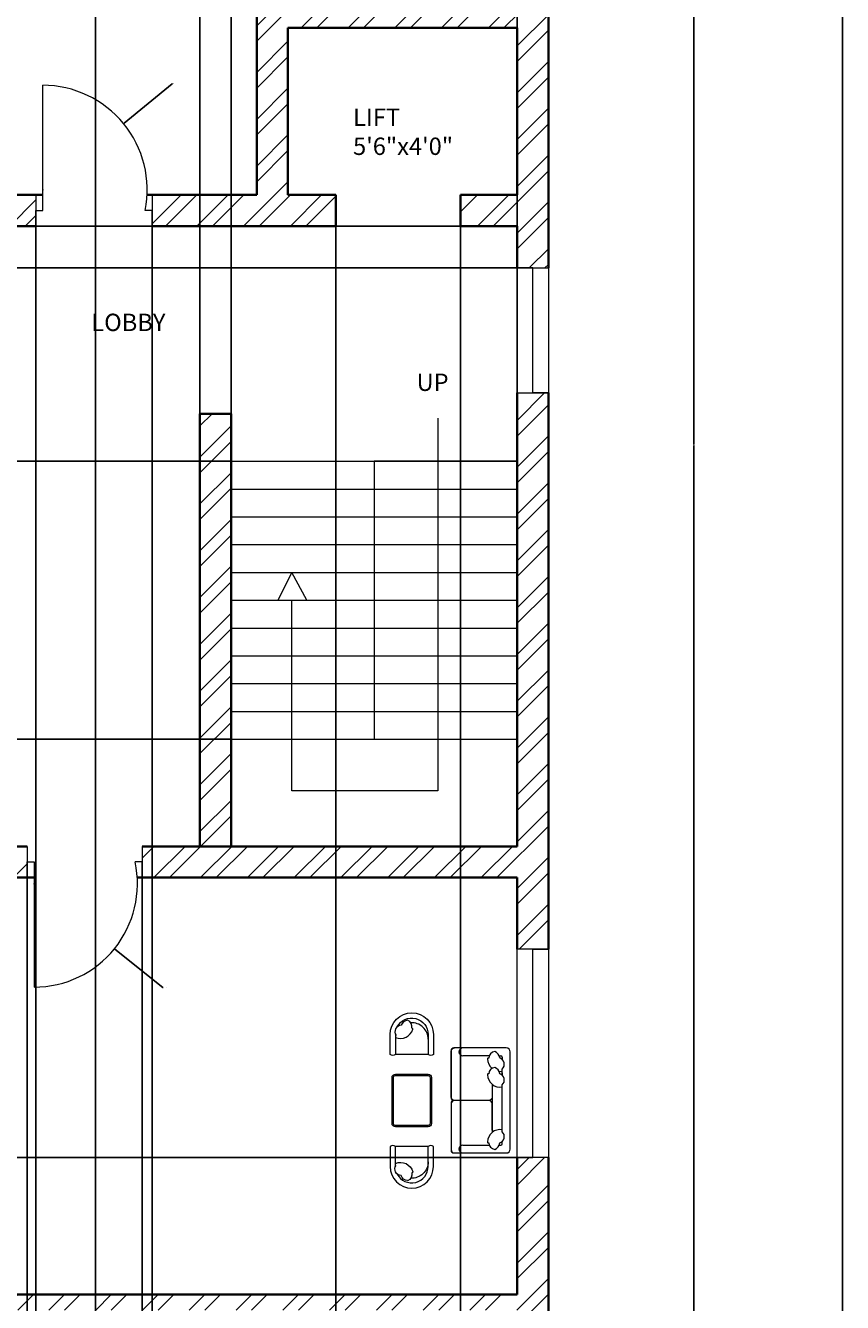
# Model space of a CAD drawing. Units: inches. Extents: x 1748 to 2382, y 1346 to 2284.
# Tile 16 of 26: x 2147 to 2382, y 1604 to 1971. Entities that reach past the tile are written whole.
import ezdxf

# ---------------------------------------------------------------- set-up
doc = ezdxf.new("R2010")
doc.units = ezdxf.units.IN
for name, color, linetype, lineweight in [('A-ANNO-DIMS', 2, 'Continuous', 18), ('A-ANNO-SYMB', 60, 'Continuous', 18), ('A-ANNO-TTLB', 7, 'Continuous', 25), ('A-AREA-IDEN', 7, 'Continuous', 18), ('A-DOOR', 21, 'Continuous', 18), ('A-FLOR-STRS', 60, 'Continuous', 18), ('A-FURN', 8, 'Continuous', 13), ('A-GLAZ', 191, 'Continuous', 18), ('A-WALL', 7, 'Continuous', 35), ('A-WALL-PATT', 9, 'Continuous', 13)]:
    doc.layers.add(name, color=color, linetype=linetype, lineweight=lineweight)
doc.styles.get("Standard").update_dxf_attribs({"font": 'arial.ttf'})
doc.dimstyles.get("Standard").update_dxf_attribs({"dimtxt": 0.18, "dimasz": 0.18, "dimexe": 0.18, "dimexo": 0.0625, "dimgap": 0.09, "dimtad": 0, "dimtih": 1, "dimtoh": 1, "dimdec": 4, "dimzin": 0, "dimdsep": 46, "dimtxsty": 'Standard', "dimcen": 0.09, "dimadec": 0, "dimazin": 0, "dimtfac": 1, "dimtdec": 4, "dimtofl": 0, "dimtmove": 0, "dimatfit": 3, "dimfxl": 1, "dimtolj": 1, "dimtzin": 0, "dimarcsym": 0})

# ---------------------------------------------------------------- blocks, each defined once
blk = doc.blocks.new('A$C1352')
at = {"color": 0}
for points in [[(0.003, 0.053), (0.003, 0.553, -0.414214), (0.053, 0.603), (0.753, 0.603, -0.414214), (0.803, 0.553), (0.803, 0.053, -0.414214), (0.753, 0.003), (0.053, 0.003, -0.414214)], [(0.023, 0.053), (0.023, 0.553, -0.414214), (0.053, 0.583), (0.753, 0.583, -0.414214), (0.783, 0.553), (0.783, 0.053, -0.414214), (0.753, 0.023), (0.053, 0.023, -0.414214)]]:
    blk.add_lwpolyline(points, format="xyb", close=True, dxfattribs=at)
blk = doc.blocks.new('WIN-60-DEEP')
for p, q in [((0, 9), (0, 0)), ((60, 9), (0, 9)), ((60, 4.5), (60, 9)), ((60, 9), (60, 0)), ((0, 0), (0, 4.5)), ((0, 4.5), (60, 4.5)), ((0, 0), (60, 0))]:
    blk.add_line(p, q)
blk = doc.blocks.new('WIN-36-DEEP')
for p, q in [((0, 9), (0, 0)), ((0, 9), (36, 9)), ((36, 4.5), (36, 9)), ((36, 9), (36, 0)), ((0, 0), (0, 4.5)), ((0, 4.5), (36, 4.5)), ((36, 0), (0, 0))]:
    blk.add_line(p, q)
blk = doc.blocks.new('CHAIR-LOUNGE')
blk.add_line((1.52, 6.05), (1.51, 0.29))
at = {"ltscale": 0.03}
blk.add_lwpolyline([(1.51, 0.29, -0.369229), (0, 0.29), (0.01, 6.05, -1), (12.48, 6.04), (12.47, 0.28, -0.369229), (10.96, 0.28)], format="xyb", close=True, dxfattribs=at)
blk.add_lwpolyline([(2.05, 8.23, -0.785087), (10.96, 6.04), (10.96, 0.28)], format="xyb")
for centre, radius, start, end in [((3.29, 6.8), 1.89, 92.9922, 214.1401), ((3, 8.54), 3.66, 247.0143, 344.2857), ((5.21, 8.01), 2.13, 94.9999, 161.3534), ((4.35, 8.32), 1.94, 346.6403, 69.4695), ((6.24, 4.71), 4.72, 359.9461, 93.658), ((6.33, 7.66), 0.226, 330.6238, 113.7423), ((6.24, 6.05), 4.72, 178.8536, 179.9461)]:
    blk.add_arc(centre, radius, start, end)
blk = doc.blocks.new('*D35')
at = {"layer": 'A-ANNO-DIMS', "color": 0, "lineweight": -2, "transparency": 16777216}
for p, q in [((2297.52, 2232.85), (2339.54, 2232.85)), ((2339.36, 2232.67), (2339.36, 1850.53)), ((2339.36, 1468.03), (2339.36, 1850.17)), ((2297.52, 1467.85), (2339.54, 1467.85))]:
    blk.add_line(p, q, dxfattribs=at)
at = {"layer": 'A-ANNO-DIMS', "color": 0, "transparency": 16777216}
for points in [[(2339.33, 2232.67), (2339.39, 2232.67), (2339.36, 2232.85)], [(2339.33, 1468.03), (2339.39, 1468.03), (2339.36, 1467.85)]]:
    blk.add_solid(points, dxfattribs=at)
at = {"layer": 'Defpoints', "color": 0, "transparency": 16777216}
for p in [(2297.46, 2232.85), (2339.36, 2232.85), (2297.46, 1467.85)]:
    blk.add_point(p, dxfattribs=at)
at = {"layer": 'A-ANNO-DIMS', "color": 0, "transparency": 16777216, "insert": (2339.36, 1850.35), "char_height": 0.18, "attachment_point": 5}
blk.add_mtext('\\A1;765', dxfattribs=at)
blk = doc.blocks.new('*D39')
at = {"layer": 'A-ANNO-DIMS', "color": 0, "lineweight": -2, "transparency": 16777216}
for p, q in [((2139.96, 1734.91), (2139.96, 2274.93)), ((2140.14, 2274.75), (2168.14, 2274.75)), ((2196.89, 2274.75), (2168.89, 2274.75)), ((2197.07, 1734.91), (2197.07, 2274.93))]:
    blk.add_line(p, q, dxfattribs=at)
at = {"layer": 'A-ANNO-DIMS', "color": 0, "transparency": 16777216}
for points in [[(2140.14, 2274.78), (2140.14, 2274.72), (2139.96, 2274.75)], [(2196.89, 2274.78), (2196.89, 2274.72), (2197.07, 2274.75)]]:
    blk.add_solid(points, dxfattribs=at)
at = {"layer": 'Defpoints', "color": 0, "transparency": 16777216}
for p in [(2197.07, 2274.75), (2139.96, 1734.85), (2197.07, 1734.85)]:
    blk.add_point(p, dxfattribs=at)
at = {"layer": 'A-ANNO-DIMS', "color": 0, "transparency": 16777216, "insert": (2168.52, 2274.75), "char_height": 0.18, "attachment_point": 5}
blk.add_mtext('\\A1;57.11', dxfattribs=at)
blk = doc.blocks.new('*D40')
at = {"layer": 'A-ANNO-DIMS', "color": 0, "lineweight": -2, "transparency": 16777216}
for p, q in [((2206.07, 1734.91), (2206.07, 2274.93)), ((2206.25, 2274.75), (2246.87, 2274.75)), ((2288.28, 2274.75), (2247.66, 2274.75)), ((2288.46, 1734.91), (2288.46, 2274.93))]:
    blk.add_line(p, q, dxfattribs=at)
at = {"layer": 'A-ANNO-DIMS', "color": 0, "transparency": 16777216}
for points in [[(2206.25, 2274.78), (2206.25, 2274.72), (2206.07, 2274.75)], [(2288.28, 2274.78), (2288.28, 2274.72), (2288.46, 2274.75)]]:
    blk.add_solid(points, dxfattribs=at)
at = {"layer": 'Defpoints', "color": 0, "transparency": 16777216}
for p in [(2288.46, 2274.75), (2206.07, 1734.85), (2288.46, 1734.85)]:
    blk.add_point(p, dxfattribs=at)
at = {"layer": 'A-ANNO-DIMS', "color": 0, "transparency": 16777216, "insert": (2247.27, 2274.75), "char_height": 0.18, "attachment_point": 5}
blk.add_mtext('\\A1;82.39', dxfattribs=at)
blk = doc.blocks.new('*D46')
at = {"layer": 'A-ANNO-DIMS', "color": 0, "lineweight": -2, "transparency": 16777216}
for p, q in [((2147.39, 1725.79), (2147.39, 1360.47)), ((2180.46, 1725.79), (2180.46, 1360.47)), ((2147.57, 1360.65), (2163.46, 1360.65)), ((2180.28, 1360.65), (2164.39, 1360.65))]:
    blk.add_line(p, q, dxfattribs=at)
at = {"layer": 'A-ANNO-DIMS', "color": 0, "transparency": 16777216}
for points in [[(2147.57, 1360.68), (2147.57, 1360.62), (2147.39, 1360.65)], [(2180.28, 1360.68), (2180.28, 1360.62), (2180.46, 1360.65)]]:
    blk.add_solid(points, dxfattribs=at)
at = {"layer": 'Defpoints', "color": 0, "transparency": 16777216}
for p in [(2147.39, 1725.85), (2180.46, 1725.85), (2180.46, 1360.65)]:
    blk.add_point(p, dxfattribs=at)
at = {"layer": 'A-ANNO-DIMS', "color": 0, "transparency": 16777216, "insert": (2163.92, 1360.65), "char_height": 0.18, "attachment_point": 5}
blk.add_mtext('\\A1;33.066', dxfattribs=at)
blk = doc.blocks.new('*D47')
at = {"layer": 'A-ANNO-DIMS', "color": 0, "lineweight": -2, "transparency": 16777216}
for p, q in [((2149.85, 1913.29), (2149.85, 1360.47)), ((2183.35, 1913.29), (2183.35, 1360.47)), ((2150.03, 1360.65), (2166.28, 1360.65)), ((2183.17, 1360.65), (2166.93, 1360.65))]:
    blk.add_line(p, q, dxfattribs=at)
at = {"layer": 'A-ANNO-DIMS', "color": 0, "transparency": 16777216}
for points in [[(2150.03, 1360.68), (2150.03, 1360.62), (2149.85, 1360.65)], [(2183.17, 1360.68), (2183.17, 1360.62), (2183.35, 1360.65)]]:
    blk.add_solid(points, dxfattribs=at)
at = {"layer": 'Defpoints', "color": 0, "transparency": 16777216}
for p in [(2149.85, 1913.35), (2183.35, 1913.35), (2183.35, 1360.65)]:
    blk.add_point(p, dxfattribs=at)
at = {"layer": 'A-ANNO-DIMS', "color": 0, "transparency": 16777216, "insert": (2166.6, 1360.65), "char_height": 0.18, "attachment_point": 5}
blk.add_mtext('\\A1;33.5', dxfattribs=at)
blk = doc.blocks.new('*D49')
at = {"layer": 'A-ANNO-DIMS', "color": 0, "lineweight": -2, "transparency": 16777216}
for p, q in [((2236.23, 1913.29), (2236.23, 1360.47)), ((2272.19, 1913.29), (2272.19, 1360.47)), ((2236.41, 1360.65), (2253.82, 1360.65)), ((2272.01, 1360.65), (2254.61, 1360.65))]:
    blk.add_line(p, q, dxfattribs=at)
at = {"layer": 'A-ANNO-DIMS', "color": 0, "transparency": 16777216}
for points in [[(2236.41, 1360.68), (2236.41, 1360.62), (2236.23, 1360.65)], [(2272.01, 1360.68), (2272.01, 1360.62), (2272.19, 1360.65)]]:
    blk.add_solid(points, dxfattribs=at)
at = {"layer": 'Defpoints', "color": 0, "transparency": 16777216}
for p in [(2236.23, 1913.35), (2272.19, 1913.35), (2272.19, 1360.65)]:
    blk.add_point(p, dxfattribs=at)
at = {"layer": 'A-ANNO-DIMS', "color": 0, "transparency": 16777216, "insert": (2254.21, 1360.65), "char_height": 0.18, "attachment_point": 5}
blk.add_mtext('\\A1;35.96', dxfattribs=at)
blk = doc.blocks.new('*D53')
at = {"layer": 'A-ANNO-DIMS', "color": 0, "lineweight": -2, "transparency": 16777216}
for p, q in [((2115.4, 2223.79), (2115.4, 1360.47)), ((2167.02, 2223.79), (2167.02, 1360.47)), ((2115.58, 1360.65), (2140.81, 1360.65)), ((2166.84, 1360.65), (2141.6, 1360.65))]:
    blk.add_line(p, q, dxfattribs=at)
at = {"layer": 'A-ANNO-DIMS', "color": 0, "transparency": 16777216}
for points in [[(2115.58, 1360.68), (2115.58, 1360.62), (2115.4, 1360.65)], [(2166.84, 1360.68), (2166.84, 1360.62), (2167.02, 1360.65)]]:
    blk.add_solid(points, dxfattribs=at)
at = {"layer": 'Defpoints', "color": 0, "transparency": 16777216}
for p in [(2115.4, 2223.85), (2167.02, 2223.85), (2167.02, 1360.65)]:
    blk.add_point(p, dxfattribs=at)
at = {"layer": 'A-ANNO-DIMS', "color": 0, "transparency": 16777216, "insert": (2141.21, 1360.65), "char_height": 0.18, "attachment_point": 5}
blk.add_mtext('\\A1;51.62', dxfattribs=at)
blk = doc.blocks.new('*D55')
at = {"layer": 'A-ANNO-DIMS', "color": 0, "lineweight": -2, "transparency": 16777216}
for p, q in [((2288.4, 1645.3), (1779.88, 1645.3)), ((1780.06, 1645.12), (1780.06, 1625.76)), ((1780.06, 1606.03), (1780.06, 1625.39)), ((2288.4, 1605.85), (1779.88, 1605.85))]:
    blk.add_line(p, q, dxfattribs=at)
at = {"layer": 'A-ANNO-DIMS', "color": 0, "transparency": 16777216}
for points in [[(1780.03, 1645.12), (1780.09, 1645.12), (1780.06, 1645.3)], [(1780.03, 1606.03), (1780.09, 1606.03), (1780.06, 1605.85)]]:
    blk.add_solid(points, dxfattribs=at)
at = {"layer": 'Defpoints', "color": 0, "transparency": 16777216}
for p in [(1780.06, 1645.3), (2288.46, 1645.3), (2288.46, 1605.85)]:
    blk.add_point(p, dxfattribs=at)
at = {"layer": 'A-ANNO-DIMS', "color": 0, "transparency": 16777216, "insert": (1780.06, 1625.58), "char_height": 0.18, "attachment_point": 5}
blk.add_mtext('\\A1;39.454', dxfattribs=at)
blk = doc.blocks.new('*D56')
at = {"layer": 'A-ANNO-DIMS', "color": 0, "lineweight": -2, "transparency": 16777216}
for p, q in [((2288.4, 1913.35), (1779.88, 1913.35)), ((1780.06, 1913.17), (1780.06, 1907.52)), ((1780.06, 1901.51), (1780.06, 1907.16)), ((2288.4, 1901.33), (1779.88, 1901.33))]:
    blk.add_line(p, q, dxfattribs=at)
at = {"layer": 'A-ANNO-DIMS', "color": 0, "transparency": 16777216}
for points in [[(1780.03, 1913.17), (1780.09, 1913.17), (1780.06, 1913.35)], [(1780.03, 1901.51), (1780.09, 1901.51), (1780.06, 1901.33)]]:
    blk.add_solid(points, dxfattribs=at)
at = {"layer": 'Defpoints', "color": 0, "transparency": 16777216}
for p in [(1780.06, 1913.35), (2288.46, 1913.35), (2288.46, 1901.33)]:
    blk.add_point(p, dxfattribs=at)
at = {"layer": 'A-ANNO-DIMS', "color": 0, "transparency": 16777216, "insert": (1780.06, 1907.34), "char_height": 0.18, "attachment_point": 5}
blk.add_mtext('\\A1;12.023', dxfattribs=at)
blk = doc.blocks.new('*D60')
at = {"layer": 'A-ANNO-DIMS', "color": 0, "lineweight": -2, "transparency": 16777216}
for p, q in [((2206.01, 1845.68), (1779.88, 1845.68)), ((1780.06, 1845.5), (1780.06, 1805.86)), ((1780.06, 1765.86), (1780.06, 1805.5)), ((2206.01, 1765.68), (1779.88, 1765.68))]:
    blk.add_line(p, q, dxfattribs=at)
at = {"layer": 'A-ANNO-DIMS', "color": 0, "transparency": 16777216}
for points in [[(1780.03, 1845.5), (1780.09, 1845.5), (1780.06, 1845.68)], [(1780.03, 1765.86), (1780.09, 1765.86), (1780.06, 1765.68)]]:
    blk.add_solid(points, dxfattribs=at)
at = {"layer": 'Defpoints', "color": 0, "transparency": 16777216}
for p in [(1780.06, 1845.68), (2206.07, 1845.68), (2206.07, 1765.68)]:
    blk.add_point(p, dxfattribs=at)
at = {"layer": 'A-ANNO-DIMS', "color": 0, "transparency": 16777216, "insert": (1780.06, 1805.68), "char_height": 0.18, "attachment_point": 5}
blk.add_mtext('\\A1;80', dxfattribs=at)
blk = doc.blocks.new('*D81')
at = {"layer": 'A-ANNO-DIMS', "color": 0, "lineweight": -2, "transparency": 16777216}
for p, q in [((2189.08, 1954.28), (2175.26, 1942.95)), ((2189.26, 1954.28), (2189.08, 1954.28)), ((2151.76, 1923.76), (2151.94, 1923.76)), ((2151.85, 1923.67), (2151.85, 1923.85))]:
    blk.add_line(p, q, dxfattribs=at)
at = {"layer": 'A-ANNO-DIMS', "color": 0, "transparency": 16777216}
blk.add_solid([(2175.24, 1942.97), (2175.28, 1942.92), (2175.12, 1942.83)], dxfattribs=at)
at = {"layer": 'Defpoints', "color": 0, "transparency": 16777216}
for p in [(2175.12, 1942.83), (2151.85, 1923.76)]:
    blk.add_point(p, dxfattribs=at)
at = {"layer": 'A-ANNO-DIMS', "color": 0, "transparency": 16777216, "insert": (2189.74, 1954.28), "char_height": 0.18, "attachment_point": 5}
blk.add_mtext('\\A1;R30.09', dxfattribs=at)
blk = doc.blocks.new('*D83')
at = {"layer": 'A-ANNO-DIMS', "color": 0, "lineweight": -2, "transparency": 16777216}
for p, q in [((2149.3, 1724.08), (2149.48, 1724.08)), ((2149.39, 1723.99), (2149.39, 1724.17)), ((2186.4, 1694.2), (2172.66, 1705.29)), ((2186.58, 1694.2), (2186.4, 1694.2))]:
    blk.add_line(p, q, dxfattribs=at)
at = {"layer": 'A-ANNO-DIMS', "color": 0, "transparency": 16777216}
blk.add_solid([(2172.68, 1705.32), (2172.65, 1705.27), (2172.52, 1705.41)], dxfattribs=at)
at = {"layer": 'Defpoints', "color": 0, "transparency": 16777216}
for p in [(2149.39, 1724.08), (2172.52, 1705.41)]:
    blk.add_point(p, dxfattribs=at)
at = {"layer": 'A-ANNO-DIMS', "color": 0, "transparency": 16777216, "insert": (2187.13, 1694.2), "char_height": 0.18, "attachment_point": 5}
blk.add_mtext('\\A1;R29.734', dxfattribs=at)

msp = doc.modelspace()

# ---------------------------------------------------------------- hatches: boundary and pattern name
at = {"layer": 'A-WALL-PATT'}
h = msp.add_hatch(dxfattribs=at)
h.set_pattern_fill('ANSI32', color=256)
h.paths.add_polyline_path([(1908.4445, 2232.8497), (1821.9607, 2232.8497), (1821.9607, 2223.8497), (1865.4607, 2223.8497), (1865.4607, 2209.9185), (1869.9607, 2209.9185), (1869.9607, 2223.8497), (1908.4445, 2223.8497), (1908.4445, 2228.3497)])
h.paths.add_polyline_path([(2040.0683, 2232.8497), (1968.4445, 2232.8497), (1968.4445, 2223.8497), (2025.9607, 2223.8497), (2025.9607, 2130.3497), (2032.1341, 2130.3497), (2032.1341, 2132.5997), (2032.1341, 2134.8497), (2030.4607, 2134.8497), (2030.4607, 2223.8497), (2040.0683, 2223.8497)])
h.paths.add_polyline_path([(2091.3969, 2232.8497), (2064.0683, 2232.8497), (2064.0683, 2223.8497), (2078.4607, 2223.8497), (2078.4607, 2134.8497), (2051.1563, 2134.8497), (2051.1563, 2130.3497), (2078.4607, 2130.3497), (2078.4607, 2128.6813), (2082.9607, 2128.6813), (2082.9607, 2130.3497), (2086.1879, 2130.3497), (2086.1879, 2132.5997), (2086.1879, 2134.8497), (2082.9607, 2134.8497), (2082.9607, 2223.8497), (2091.3969, 2223.8497), (2091.3969, 2228.3497)])
h.paths.add_polyline_path([(2167.0164, 2232.8497), (2115.3969, 2232.8497), (2115.3969, 2223.8497), (2130.9607, 2223.8497), (2130.9607, 2134.8497), (2106.9607, 2134.8497), (2106.9607, 2130.3497), (2135.4607, 2130.3497), (2135.4607, 2223.8497), (2167.0164, 2223.8497), (2167.0164, 2228.3497)])
h.paths.add_polyline_path([(1869.9607, 2149.9185), (1865.4607, 2149.9185), (1865.4607, 2127.8942), (1869.9607, 2127.8942)])
h.paths.add_polyline_path([(2082.9607, 2104.4871), (2080.7107, 2104.4871), (2078.4607, 2104.4871), (2078.4607, 2103.8497), (1869.9607, 2103.8497), (1869.9607, 2108.6062), (1867.7107, 2108.6062), (1865.4607, 2108.6062), (1865.4607, 2103.8497), (1821.9607, 2103.8497), (1821.9607, 2099.3497), (1865.4607, 2099.3497), (1865.4607, 2094.7509), (1869.9607, 2094.7509), (1869.9607, 2099.3497), (2025.9607, 2099.3497), (2025.9607, 2096.4326), (2030.4607, 2096.4326), (2030.4607, 2099.3497), (2082.9607, 2099.3497)])
h.paths.add_polyline_path([(1928.9457, 1401.1212), (2176.8693, 1401.1212), (2176.8693, 1438.214), (1928.9457, 1438.214)], flags=9)
h.paths.add_polyline_path([(2122.2668, 2048.1927), (2177.9387, 2048.1927), (2177.9387, 2066.85), (2122.2668, 2066.85)], flags=9)
h.paths.add_polyline_path([(2272.688, 2153.8197), (2272.688, 2216.746), (2262.3845, 2216.746), (2262.3845, 2153.8197)], flags=9)
h.paths.add_polyline_path([(2157.2928, 2166.5593), (2196.3822, 2166.5593), (2196.3822, 2185.2167), (2157.2928, 2185.2167)], flags=9)
h.paths.add_polyline_path([(2089.3407, 2162.0698), (2124.3987, 2162.0698), (2124.3987, 2180.7272), (2089.3407, 2180.7272)], flags=9)
h.paths.add_polyline_path([(2037.4521, 2160.0913), (2072.5101, 2160.0913), (2072.5101, 2178.7486), (2037.4521, 2178.7486)], flags=9)
h.paths.add_polyline_path([(1884.7894, 2104.1554), (1923.6297, 2104.1554), (1923.6297, 2122.8127), (1884.7894, 2122.8127)], flags=9)
h.paths.add_polyline_path([(1851.2832, 2142.9749), (1851.2832, 2199.3051), (1840.9796, 2199.3051), (1840.9796, 2142.9749)], flags=9)
h.paths.add_polyline_path([(1844.8763, 2017.2834), (1844.8763, 2073.6136), (1834.5728, 2073.6136), (1834.5728, 2017.2834)], flags=9)
h.paths.add_polyline_path([(1897.1577, 2073.1279), (1935.9981, 2073.1279), (1935.9981, 2091.7853), (1897.1577, 2091.7853)], flags=9)
h.paths.add_polyline_path([(1952.3395, 1802.4231), (2008.0114, 1802.4231), (2008.0114, 1821.0805), (1952.3395, 1821.0805)], flags=9)
h.paths.add_polyline_path([(1978.8184, 1857.6841), (2017.7338, 1857.6841), (2017.7338, 1876.3415), (1978.8184, 1876.3415)], flags=9)
h.paths.add_polyline_path([(1979.6513, 1925.9516), (2008.8089, 1925.9516), (2008.8089, 1944.6089), (1979.6513, 1944.6089)], flags=9)
h.paths.add_polyline_path([(1838.5553, 1860.3527), (1877.3957, 1860.3527), (1877.3957, 1879.01), (1838.5553, 1879.01)], flags=9)
h.paths.add_polyline_path([(1883.9018, 1787.3013), (1883.9018, 1843.6315), (1873.5983, 1843.6315), (1873.5983, 1787.3013)], flags=9)
h.paths.add_polyline_path([(1873.7079, 1509.1938), (1873.7079, 1583.7709), (1863.4044, 1583.7709), (1863.4044, 1509.1938)], flags=9)
h.paths.add_polyline_path([(1916.2259, 1603.3681), (1955.0663, 1603.3681), (1955.0663, 1622.0254), (1916.2259, 1622.0254)], flags=9)
h.paths.add_polyline_path([(1876.3013, 1636.757), (1876.3013, 1693.0871), (1865.9978, 1693.0871), (1865.9978, 1636.757)], flags=9)
h.paths.add_polyline_path([(1921.3138, 1521.8316), (1964.0662, 1521.8316), (1964.0662, 1540.489), (1921.3138, 1540.489)], flags=9)
h.paths.add_polyline_path([(2017.5657, 1497.5078), (2046.7983, 1497.5078), (2046.7983, 1516.1651), (2017.5657, 1516.1651)], flags=9)
h.paths.add_polyline_path([(2066.8661, 1499.3902), (2096.0988, 1499.3902), (2096.0988, 1518.0475), (2066.8661, 1518.0475)], flags=9)
h.paths.add_polyline_path([(2155.4835, 1571.6596), (2198.2358, 1571.6596), (2198.2358, 1590.3169), (2155.4835, 1590.3169)], flags=9)
h.paths.add_polyline_path([(2094.9136, 1664.6812), (2150.5855, 1664.6812), (2150.5855, 1683.3386), (2094.9136, 1683.3386)], flags=9)
h.paths.add_polyline_path([(2257.6902, 1863.1628), (2269.8935, 1863.1628), (2269.8935, 1873.4664), (2257.6902, 1873.4664)], flags=9)
h.paths.add_polyline_path([(2164.0748, 1880.3089), (2189.8694, 1880.3089), (2189.8694, 1890.6124), (2164.0748, 1890.6124)], flags=9)
h.paths.add_polyline_path([(2239.4394, 1931.0585), (2268.8187, 1931.0585), (2268.8187, 1949.7159), (2239.4394, 1949.7159)], flags=9)
h = msp.add_hatch(dxfattribs=at)
h.set_pattern_fill('ANSI32', color=256)
h.paths.add_polyline_path([(2297.4607, 2232.8497), (2203.0164, 2232.8497), (2203.0164, 2223.8497), (2244.9607, 2223.8497), (2244.9607, 2127.8554), (2249.4607, 2127.8554), (2249.4607, 2223.8497), (2297.4607, 2223.8497)])
h.paths.add_polyline_path([(2297.4607, 2103.8497), (2249.4607, 2103.8497), (2249.4607, 2106.7497), (2247.2107, 2106.7497), (2244.9607, 2106.7497), (2244.9607, 2103.8497), (2130.9607, 2103.8497), (2130.9607, 2099.3497), (2288.4607, 2099.3497), (2288.4607, 2077.2008), (2297.4607, 2077.2008)])
h.paths.add_polyline_path([(1928.9457, 1401.1212), (2176.8693, 1401.1212), (2176.8693, 1438.214), (1928.9457, 1438.214)], flags=9)
h.paths.add_polyline_path([(2122.2668, 2048.1927), (2177.9387, 2048.1927), (2177.9387, 2066.85), (2122.2668, 2066.85)], flags=9)
h.paths.add_polyline_path([(2272.688, 2153.8197), (2272.688, 2216.746), (2262.3845, 2216.746), (2262.3845, 2153.8197)], flags=25)
h.paths.add_polyline_path([(2157.2928, 2166.5593), (2196.3822, 2166.5593), (2196.3822, 2185.2167), (2157.2928, 2185.2167)], flags=9)
h.paths.add_polyline_path([(2089.3407, 2162.0698), (2124.3987, 2162.0698), (2124.3987, 2180.7272), (2089.3407, 2180.7272)], flags=9)
h.paths.add_polyline_path([(2037.4521, 2160.0913), (2072.5101, 2160.0913), (2072.5101, 2178.7486), (2037.4521, 2178.7486)], flags=9)
h.paths.add_polyline_path([(1884.7894, 2104.1554), (1923.6297, 2104.1554), (1923.6297, 2122.8127), (1884.7894, 2122.8127)], flags=9)
h.paths.add_polyline_path([(1851.2832, 2142.9749), (1851.2832, 2199.3051), (1840.9796, 2199.3051), (1840.9796, 2142.9749)], flags=9)
h.paths.add_polyline_path([(1844.8763, 2017.2834), (1844.8763, 2073.6136), (1834.5728, 2073.6136), (1834.5728, 2017.2834)], flags=9)
h.paths.add_polyline_path([(1897.1577, 2073.1279), (1935.9981, 2073.1279), (1935.9981, 2091.7853), (1897.1577, 2091.7853)], flags=9)
h.paths.add_polyline_path([(1952.3395, 1802.4231), (2008.0114, 1802.4231), (2008.0114, 1821.0805), (1952.3395, 1821.0805)], flags=9)
h.paths.add_polyline_path([(1978.8184, 1857.6841), (2017.7338, 1857.6841), (2017.7338, 1876.3415), (1978.8184, 1876.3415)], flags=9)
h.paths.add_polyline_path([(1979.6513, 1925.9516), (2008.8089, 1925.9516), (2008.8089, 1944.6089), (1979.6513, 1944.6089)], flags=9)
h.paths.add_polyline_path([(1838.5553, 1860.3527), (1877.3957, 1860.3527), (1877.3957, 1879.01), (1838.5553, 1879.01)], flags=9)
h.paths.add_polyline_path([(1883.9018, 1787.3013), (1883.9018, 1843.6315), (1873.5983, 1843.6315), (1873.5983, 1787.3013)], flags=9)
h.paths.add_polyline_path([(1873.7079, 1509.1938), (1873.7079, 1583.7709), (1863.4044, 1583.7709), (1863.4044, 1509.1938)], flags=9)
h.paths.add_polyline_path([(1916.2259, 1603.3681), (1955.0663, 1603.3681), (1955.0663, 1622.0254), (1916.2259, 1622.0254)], flags=9)
h.paths.add_polyline_path([(1876.3013, 1636.757), (1876.3013, 1693.0871), (1865.9978, 1693.0871), (1865.9978, 1636.757)], flags=9)
h.paths.add_polyline_path([(1921.3138, 1521.8316), (1964.0662, 1521.8316), (1964.0662, 1540.489), (1921.3138, 1540.489)], flags=9)
h.paths.add_polyline_path([(2017.5657, 1497.5078), (2046.7983, 1497.5078), (2046.7983, 1516.1651), (2017.5657, 1516.1651)], flags=9)
h.paths.add_polyline_path([(2066.8661, 1499.3902), (2096.0988, 1499.3902), (2096.0988, 1518.0475), (2066.8661, 1518.0475)], flags=9)
h.paths.add_polyline_path([(2155.4835, 1571.6596), (2198.2358, 1571.6596), (2198.2358, 1590.3169), (2155.4835, 1590.3169)], flags=9)
h.paths.add_polyline_path([(2094.9136, 1664.6812), (2150.5855, 1664.6812), (2150.5855, 1683.3386), (2094.9136, 1683.3386)], flags=9)
h.paths.add_polyline_path([(2257.6902, 1863.1628), (2269.8935, 1863.1628), (2269.8935, 1873.4664), (2257.6902, 1873.4664)], flags=9)
h.paths.add_polyline_path([(2164.0748, 1880.3089), (2189.8694, 1880.3089), (2189.8694, 1890.6124), (2164.0748, 1890.6124)], flags=9)
h.paths.add_polyline_path([(2239.4394, 1931.0585), (2268.8187, 1931.0585), (2268.8187, 1949.7159), (2239.4394, 1949.7159)], flags=9)
h = msp.add_hatch(dxfattribs=at)
h.set_pattern_fill('ANSI32', color=256)
h.paths.add_polyline_path([(1919.6777, 1476.8497), (1900.6426, 1476.8497), (1900.6426, 1522.0826), (1898.3926, 1522.0826), (1896.1426, 1522.0826), (1896.1426, 1476.8497), (1857.1426, 1476.8497), (1857.1426, 1467.8497), (1896.1426, 1467.8497), (1919.6777, 1467.8497), (1919.6777, 1472.3497)])
h.paths.add_polyline_path([(2018.7873, 1472.3497), (2018.7873, 1476.8497), (2010.9607, 1476.8497), (2010.9607, 1560.8497), (2034.9607, 1560.8497), (2034.9607, 1565.3497), (2006.4607, 1565.3497), (2006.4607, 1476.8497), (1955.6777, 1476.8497), (1955.6777, 1467.8497), (2018.7873, 1467.8497)])
h.paths.add_polyline_path([(2152.3354, 1472.3497), (2152.3354, 1476.8497), (2115.9607, 1476.8497), (2115.9607, 1565.3497), (2109.2204, 1565.3497), (2109.2204, 1563.0997), (2109.2204, 1560.8497), (2111.4607, 1560.8497), (2111.4607, 1476.8497), (2095.3617, 1476.8497), (2095.3617, 1467.8497), (2152.3354, 1467.8497)])
h.paths.add_polyline_path([(2071.3617, 1476.8497), (2063.4607, 1476.8497), (2063.4607, 1560.8497), (2090.1865, 1560.8497), (2090.1865, 1565.3497), (2063.4607, 1565.3497), (2063.4607, 1572.5485), (2061.2107, 1572.5485), (2058.9607, 1572.5485), (2058.9607, 1565.3497), (2055.6281, 1565.3497), (2055.6281, 1560.8497), (2058.9607, 1560.8497), (2058.9607, 1476.8497), (2042.7873, 1476.8497), (2042.7873, 1467.8497), (2071.3617, 1467.8497), (2071.3617, 1472.3497)])
h.paths.add_polyline_path([(2297.4607, 1506.5652), (2288.4607, 1506.5652), (2288.4607, 1476.8497), (2212.3354, 1476.8497), (2212.3354, 1467.8497), (2297.4607, 1467.8497)])
h.paths.add_polyline_path([(2297.4607, 1645.3038), (2288.4607, 1645.3038), (2288.4607, 1605.8497), (2058.9607, 1605.8497), (2058.9607, 1600.1857), (2061.2107, 1600.1857), (2063.4607, 1600.1857), (2063.4607, 1601.3497), (2288.4607, 1601.3497), (2288.4607, 1566.5652), (2297.4607, 1566.5652)])
h.paths.add_polyline_path([(2010.9607, 1609.0561), (2008.7107, 1609.0561), (2006.4607, 1609.0561), (2006.4607, 1605.8497), (1900.6426, 1605.8497), (1900.6426, 1609.7171), (1898.3926, 1609.7171), (1896.1426, 1609.7171), (1896.1426, 1605.8497), (1857.1426, 1605.8497), (1857.1426, 1601.3497), (1896.1426, 1601.3497), (1896.1426, 1542.5447), (1900.6426, 1542.5447), (1900.6426, 1601.3497), (2010.9607, 1601.3497)])
h.paths.add_polyline_path([(1928.9457, 1401.1212), (2176.8693, 1401.1212), (2176.8693, 1438.214), (1928.9457, 1438.214)], flags=9)
h.paths.add_polyline_path([(2122.2668, 2048.1927), (2177.9387, 2048.1927), (2177.9387, 2066.85), (2122.2668, 2066.85)], flags=9)
h.paths.add_polyline_path([(2272.688, 2153.8197), (2272.688, 2216.746), (2262.3845, 2216.746), (2262.3845, 2153.8197)], flags=9)
h.paths.add_polyline_path([(2157.2928, 2166.5593), (2196.3822, 2166.5593), (2196.3822, 2185.2167), (2157.2928, 2185.2167)], flags=9)
h.paths.add_polyline_path([(2089.3407, 2162.0698), (2124.3987, 2162.0698), (2124.3987, 2180.7272), (2089.3407, 2180.7272)], flags=9)
h.paths.add_polyline_path([(2037.4521, 2160.0913), (2072.5101, 2160.0913), (2072.5101, 2178.7486), (2037.4521, 2178.7486)], flags=9)
h.paths.add_polyline_path([(1884.7894, 2104.1554), (1923.6297, 2104.1554), (1923.6297, 2122.8127), (1884.7894, 2122.8127)], flags=9)
h.paths.add_polyline_path([(1851.2832, 2142.9749), (1851.2832, 2199.3051), (1840.9796, 2199.3051), (1840.9796, 2142.9749)], flags=9)
h.paths.add_polyline_path([(1844.8763, 2017.2834), (1844.8763, 2073.6136), (1834.5728, 2073.6136), (1834.5728, 2017.2834)], flags=9)
h.paths.add_polyline_path([(1897.1577, 2073.1279), (1935.9981, 2073.1279), (1935.9981, 2091.7853), (1897.1577, 2091.7853)], flags=9)
h.paths.add_polyline_path([(1952.3395, 1802.4231), (2008.0114, 1802.4231), (2008.0114, 1821.0805), (1952.3395, 1821.0805)], flags=9)
h.paths.add_polyline_path([(1978.8184, 1857.6841), (2017.7338, 1857.6841), (2017.7338, 1876.3415), (1978.8184, 1876.3415)], flags=9)
h.paths.add_polyline_path([(1979.6513, 1925.9516), (2008.8089, 1925.9516), (2008.8089, 1944.6089), (1979.6513, 1944.6089)], flags=9)
h.paths.add_polyline_path([(1838.5553, 1860.3527), (1877.3957, 1860.3527), (1877.3957, 1879.01), (1838.5553, 1879.01)], flags=9)
h.paths.add_polyline_path([(1883.9018, 1787.3013), (1883.9018, 1843.6315), (1873.5983, 1843.6315), (1873.5983, 1787.3013)], flags=9)
h.paths.add_polyline_path([(1873.7079, 1509.1938), (1873.7079, 1583.7709), (1863.4044, 1583.7709), (1863.4044, 1509.1938)], flags=9)
h.paths.add_polyline_path([(1916.2259, 1603.3681), (1955.0663, 1603.3681), (1955.0663, 1622.0254), (1916.2259, 1622.0254)], flags=9)
h.paths.add_polyline_path([(1876.3013, 1636.757), (1876.3013, 1693.0871), (1865.9978, 1693.0871), (1865.9978, 1636.757)], flags=9)
h.paths.add_polyline_path([(1921.3138, 1521.8316), (1964.0662, 1521.8316), (1964.0662, 1540.489), (1921.3138, 1540.489)], flags=9)
h.paths.add_polyline_path([(2017.5657, 1497.5078), (2046.7983, 1497.5078), (2046.7983, 1516.1651), (2017.5657, 1516.1651)], flags=9)
h.paths.add_polyline_path([(2066.8661, 1499.3902), (2096.0988, 1499.3902), (2096.0988, 1518.0475), (2066.8661, 1518.0475)], flags=9)
h.paths.add_polyline_path([(2155.4835, 1571.6596), (2198.2358, 1571.6596), (2198.2358, 1590.3169), (2155.4835, 1590.3169)], flags=25)
h.paths.add_polyline_path([(2094.9136, 1664.6812), (2150.5855, 1664.6812), (2150.5855, 1683.3386), (2094.9136, 1683.3386)], flags=9)
h.paths.add_polyline_path([(2257.6902, 1863.1628), (2269.8935, 1863.1628), (2269.8935, 1873.4664), (2257.6902, 1873.4664)], flags=9)
h.paths.add_polyline_path([(2164.0748, 1880.3089), (2189.8694, 1880.3089), (2189.8694, 1890.6124), (2164.0748, 1890.6124)], flags=9)
h.paths.add_polyline_path([(2239.4394, 1931.0585), (2268.8187, 1931.0585), (2268.8187, 1949.7159), (2239.4394, 1949.7159)], flags=9)
h = msp.add_hatch(dxfattribs=at)
h.set_pattern_fill('ANSI32', color=256)
h.paths.add_polyline_path([(1900.6426, 1652.723), (1896.1426, 1652.723), (1896.1426, 1629.9029), (1900.6426, 1629.9029)])
h.paths.add_polyline_path([(2206.0699, 1859.3497), (2197.0699, 1859.3497), (2197.0699, 1734.8497), (2206.0699, 1734.8497)], flags=17)
h.paths.add_polyline_path([(2297.4607, 1865.3269), (2288.4607, 1865.3269), (2288.4607, 1734.8497), (2206.0699, 1734.8497), (2180.4551, 1734.8497), (2180.4551, 1725.8497), (2197.0699, 1725.8497), (2206.0699, 1725.8497), (2288.4607, 1725.8497), (2288.4607, 1705.3038), (2297.4607, 1705.3038)])
h.paths.add_polyline_path([(2139.9607, 1815.8001), (2135.4607, 1815.8001), (2130.9607, 1815.8001), (2130.9607, 1734.8497), (1900.6426, 1734.8497), (1900.6426, 1738.9477), (1898.3926, 1738.9477), (1896.1426, 1738.9477), (1896.1426, 1734.8497), (1857.1426, 1734.8497), (1857.1426, 1725.8497), (1896.1426, 1725.8497), (1896.1426, 1712.723), (1900.6426, 1712.723), (1900.6426, 1725.8497), (2006.4607, 1725.8497), (2006.4607, 1637.448), (2010.9607, 1637.448), (2010.9607, 1725.8497), (2139.9607, 1725.8497), (2147.389, 1725.8497), (2147.389, 1730.3497), (2147.389, 1734.8497), (2139.9607, 1734.8497)])
h.paths.add_polyline_path([(2149.8497, 1917.8497), (2149.8497, 1922.3497), (2139.9607, 1922.3497), (2139.9607, 1979.3497), (2030.4607, 1979.3497), (2030.4607, 2069.8971), (2028.2107, 2069.8971), (2025.9607, 2069.8971), (2025.9607, 1979.3497), (1869.9607, 1979.3497), (1869.9607, 1998.93), (1865.4607, 1998.93), (1865.4607, 1979.3497), (1821.9607, 1979.3497), (1821.9607, 1952.7922), (1826.9306, 1952.7922), (1830.9607, 1952.7922), (1830.9607, 1970.3497), (1962.9607, 1970.3497), (1962.9607, 1926.5713), (1967.4607, 1926.5713), (1967.4607, 1970.3497), (2027.4607, 1970.3497), (2027.4607, 1898.3497), (2004.9604, 1898.3497), (2004.9604, 1893.8497), (2027.4607, 1893.8497), (2027.4607, 1859.3497), (1958.8973, 1859.3497), (1958.8973, 1854.8497), (2047.917, 1854.8497), (2047.917, 1859.3497), (2031.9607, 1859.3497), (2031.9607, 1970.3497), (2130.9607, 1970.3497), (2130.9607, 1859.3497), (2104.9565, 1859.3497), (2104.9565, 1854.8497), (2130.9607, 1854.8497), (2130.9607, 1849.0684), (2139.9607, 1849.0684), (2139.9607, 1913.3497), (2149.8497, 1913.3497)])
h.paths.add_polyline_path([(1928.9996, 1859.3497), (1830.9607, 1859.3497), (1830.9607, 1892.7922), (1821.9607, 1892.7922), (1821.9607, 1854.8497), (1896.1426, 1854.8497), (1896.1426, 1836.6443), (1898.378, 1836.6443), (1900.6426, 1836.6443), (1900.6426, 1854.8497), (1928.9996, 1854.8497), (1928.9996, 1857.0997)])
h.paths.add_polyline_path([(1980.9604, 1896.0997), (1980.9604, 1898.3497), (1967.4607, 1898.3497), (1967.4607, 1902.3846), (1962.9607, 1902.3846), (1962.9607, 1859.3497), (1967.4607, 1859.3497), (1967.4607, 1893.8497), (1980.9604, 1893.8497)], flags=17)
h.paths.add_polyline_path([(1900.6426, 1776.6443), (1896.1426, 1776.6443), (1896.1426, 1758.0891), (1900.6426, 1758.0891)], flags=17)
h.paths.add_polyline_path([(2297.4607, 2017.2008), (2288.4607, 2017.2008), (2288.4607, 1979.3497), (2213.4607, 1979.3497), (2213.4607, 1922.3497), (2183.3516, 1922.3497), (2183.3516, 1913.3497), (2213.4607, 1913.3497), (2236.234, 1913.3497), (2236.234, 1922.3497), (2222.4607, 1922.3497), (2222.4607, 1931.3497), (2222.4607, 1970.3497), (2288.4607, 1970.3497), (2288.4607, 1922.3497), (2272.1921, 1922.3497), (2272.1921, 1913.3497), (2288.4607, 1913.3497), (2288.4607, 1901.3269), (2297.4607, 1901.3269)])

# ---------------------------------------------------------------- linework, layer by layer
at = {"layer": 'A-ANNO-SYMB'}
for p, q in [((2265.578, 1858.1104), (2265.578, 1750.8005)), ((2223.5719, 1813.6799), (2219.595, 1805.6799)), ((2227.9327, 1805.6799), (2223.5719, 1813.6799)), ((2219.595, 1805.6799), (2227.9327, 1805.6799)), ((2223.5719, 1750.8005), (2223.5719, 1805.6799)), ((2265.578, 1750.8005), (2223.5719, 1750.8005))]:
    msp.add_line(p, q, dxfattribs=at)
at = {"layer": 'A-ANNO-TTLB'}
msp.add_lwpolyline([(1747.8112, 2284.3704), (2382.1361, 2284.3704), (2382.1361, 1346.4899), (1747.8112, 1346.4899)], close=True, dxfattribs=at)
at = {"layer": 'A-DOOR'}
for p, q in [((2151.8497, 1917.8497), (2151.8497, 1953.8497)), ((2149.8497, 1922.3497), (2149.8497, 1913.3497)), ((2183.3516, 1922.3497), (2183.3516, 1913.3497)), ((2149.8497, 1913.3497), (2149.8497, 1917.8497)), ((2149.8497, 1917.8497), (2151.8497, 1917.8497)), ((2183.3516, 1917.8497), (2181.3516, 1917.8497)), ((2183.3516, 1913.3497), (2183.3516, 1917.8497)), ((2147.389, 1734.8497), (2147.389, 1725.8497)), ((2180.4551, 1734.8497), (2180.4551, 1725.8497)), ((2147.389, 1725.8497), (2147.389, 1730.3497)), ((2147.389, 1730.3497), (2149.389, 1730.3497)), ((2149.389, 1730.3497), (2149.389, 1694.3497)), ((2180.4551, 1730.3497), (2178.4551, 1730.3497)), ((2180.4551, 1725.8497), (2180.4551, 1730.3497))]:
    msp.add_line(p, q, dxfattribs=at)
for centre, radius, start, end in [((2151.8497, 1923.7612), 30.0884, 348.669155, 90), ((2149.389, 1724.0835), 29.7338, 270, 12.165865)]:
    msp.add_arc(centre, radius, start, end, dxfattribs=at)
at = {"layer": 'A-FLOR-STRS'}
for p, q in [((2206.0699, 1845.6799), (2288.4607, 1845.6799)), ((2288.4607, 1845.6799), (2247.2653, 1845.6799)), ((2247.2653, 1845.6799), (2247.2653, 1765.6799)), ((2206.0699, 1837.6799), (2288.4607, 1837.6799)), ((2206.0699, 1829.6799), (2288.4607, 1829.6799)), ((2206.0699, 1821.6799), (2288.4607, 1821.6799)), ((2206.0699, 1813.6799), (2288.4607, 1813.6799)), ((2206.0699, 1805.6799), (2288.4607, 1805.6799)), ((2206.0699, 1797.6799), (2288.4607, 1797.6799)), ((2206.0699, 1789.6799), (2288.4607, 1789.6799)), ((2206.0699, 1781.6799), (2288.4607, 1781.6799)), ((2206.0699, 1773.6799), (2288.4607, 1773.6799)), ((2206.0699, 1765.6799), (2288.4607, 1765.6799))]:
    msp.add_line(p, q, dxfattribs=at)
at = {"layer": 'A-FURN'}
for p, q in [((2280.4131, 1674.5751), (2272.8483, 1674.5751)), ((2283.2814, 1674.5751), (2283.8076, 1674.5751)), ((2284.1855, 1674.1972), (2284.1855, 1673.502)), ((2284.1855, 1668.9654), (2284.1855, 1670.7738)), ((2284.1855, 1669.6606), (2284.1855, 1668.9654)), ((2284.1855, 1652.6788), (2284.1855, 1666.2373)), ((2284.1855, 1649.2554), (2284.1855, 1649.9507)), ((2272.8483, 1648.8775), (2280.4131, 1648.8775)), ((2283.2814, 1648.8775), (2283.8076, 1648.8775))]:
    msp.add_line(p, q, dxfattribs=at)
at = {"layer": 'A-FURN', "ltscale": 0.03}
msp.add_lwpolyline([(2270.203, 1661.717, 0.41421356), (2269.4471, 1660.9612), (2269.4471, 1647.3659, 0.41421356), (2270.203, 1646.6101), (2285.3192, 1646.6101, 0.41421356), (2286.4529, 1647.7438), (2286.4529, 1675.7088, 0.41421356), (2285.3192, 1676.8426), (2270.203, 1676.8426, 0.41421356), (2269.4471, 1676.0867), (2269.4471, 1662.4914, 0.41421356), (2270.203, 1661.7356)], format="xyb", dxfattribs=at)
at = {"layer": 'A-FURN'}
for points in [[(2281.2567, 1666.3889), (2281.2567, 1662.6711, -0.41421356), (2280.3119, 1661.7263), (2270.3919, 1661.7263, -0.41421356), (2269.4471, 1662.6711), (2269.4471, 1675.8978, -0.41421356), (2270.3919, 1676.8426)], [(2281.2567, 1653.1706), (2281.2567, 1660.7816, 0.41421356), (2280.3119, 1661.7263), (2270.3919, 1661.7263, 0.41421356), (2269.4471, 1660.7816), (2269.4471, 1647.5549, 0.41421356), (2270.3919, 1646.6101)]]:
    msp.add_lwpolyline(points, format="xyb", dxfattribs=at)
msp.add_lwpolyline([(2281.2567, 1666.3889), (2281.2567, 1652.5272)], dxfattribs=at)
for centre, radius, start, end in [((2272.8483, 1675.7088), 1.1337, 90, 180), ((2272.8483, 1675.7088), 1.1337, 180, 270), ((2282.2195, 1673.8628), 1.9418, 96.427858, 179.256998), ((2281.3047, 1673.7787), 2.1311, 4.543938, 70.89739), ((2280.1392, 1673.7095), 0.226, 52.154994, 195.27353), ((2283.5777, 1673.7528), 3.658, 181.611631, 229.375991), ((2282.8726, 1672.1379), 1.8933, 311.757236, 72.905096), ((2283.8076, 1674.1972), 0.3779, 0, 90), ((2283.8076, 1674.1972), 0.3779, 0, 90), ((2280.1392, 1669.1729), 0.226, 52.154994, 195.27353), ((2283.5777, 1669.2163), 3.658, 181.611631, 278.88305), ((2282.2195, 1669.3263), 1.9418, 96.427858, 179.256998), ((2281.3047, 1669.2421), 2.1311, 4.543938, 70.89739), ((2283.5777, 1673.7528), 3.658, 264.880983, 278.88305), ((2282.8726, 1667.6013), 1.8933, 311.757236, 72.905096), ((2283.5777, 1649.6998), 3.658, 81.11695, 178.388369), ((2282.8726, 1651.3147), 1.8933, 287.094904, 48.242764), ((2272.8483, 1647.7438), 1.1337, 90, 180), ((2272.8483, 1647.7438), 1.1337, 180, 270), ((2280.1392, 1649.7431), 0.226, 164.72647, 307.845006), ((2282.2195, 1649.5898), 1.9418, 180.743002, 263.572142), ((2281.3047, 1649.674), 2.1311, 289.10261, 355.456062), ((2283.8076, 1649.2554), 0.3779, 270, 0)]:
    msp.add_arc(centre, radius, start, end, dxfattribs=at)
at = {"layer": 'A-WALL'}
for p, q in [((2297.4607, 2017.2008), (2297.4607, 1901.3269)), ((2213.4607, 1979.3497), (2213.4607, 1922.3497)), ((2222.4607, 1970.3497), (2222.4607, 1931.3497)), ((2288.4607, 1970.3497), (2222.4607, 1970.3497)), ((2288.4607, 1970.3497), (2288.4607, 1922.3497)), ((2222.4607, 1931.3497), (2222.4607, 1922.3497)), ((2139.9607, 1922.3497), (2151.8497, 1922.3497)), ((2181.9049, 1922.3497), (2213.4607, 1922.3497)), ((2222.4607, 1922.3497), (2236.234, 1922.3497)), ((2236.234, 1922.3497), (2236.234, 1913.3497)), ((2272.1921, 1922.3497), (2272.1921, 1913.3497)), ((2272.1921, 1922.3497), (2288.4607, 1922.3497)), ((2149.8497, 1913.3497), (2139.9607, 1913.3497)), ((2213.4607, 1913.3497), (2183.3516, 1913.3497)), ((2213.4607, 1913.3497), (2236.234, 1913.3497)), ((2272.1921, 1913.3497), (2288.4607, 1913.3497)), ((2288.4607, 1913.3497), (2288.4607, 1901.3269)), ((2288.4607, 1865.3269), (2288.4607, 1734.8497)), ((2297.4607, 1865.3269), (2297.4607, 1705.3038)), ((2197.0699, 1859.3497), (2206.0699, 1859.3497)), ((2197.0699, 1859.3497), (2197.0699, 1734.8497)), ((2206.0699, 1734.8497), (2206.0699, 1859.3497)), ((2147.389, 1734.8497), (2139.9607, 1734.8497)), ((2206.0699, 1734.8497), (2180.4551, 1734.8497)), ((2206.0699, 1734.8497), (2288.4607, 1734.8497)), ((2139.9607, 1725.8497), (2149.389, 1725.8497)), ((2179.0704, 1725.8497), (2197.0699, 1725.8497)), ((2197.0699, 1725.8497), (2206.0699, 1725.8497)), ((2197.0699, 1725.8497), (2288.4607, 1725.8497)), ((2288.4607, 1725.8497), (2288.4607, 1705.3038)), ((2288.4607, 1645.3038), (2288.4607, 1605.8497)), ((2297.4607, 1645.3038), (2297.4607, 1566.5652)), ((2058.9607, 1605.8497), (2288.4607, 1605.8497))]:
    msp.add_line(p, q, dxfattribs=at)

# ---------------------------------------------------------------- block references
at = {"layer": 'A-FURN'}
msp.add_blockref('CHAIR-LOUNGE', (2251.8742, 1674.6692), dxfattribs=at)
at = {"layer": 'A-FURN', "ltscale": 0.03, "xscale": 18.89529246734385, "yscale": 18.89529246734385, "zscale": 18.89529246734385, "rotation": 270}
msp.add_blockref('A$C1352', (2252.3848, 1669.3352), dxfattribs=at)
at = {"layer": 'A-FURN', "extrusion": (0, 0, -1), "zscale": -1, "rotation": 180}
msp.add_blockref('CHAIR-LOUNGE', (-2251.8742, 1648.7835), dxfattribs=at)
at = {"layer": 'A-GLAZ', "rotation": 90}
msp.add_blockref('WIN-36-DEEP', (2297.4603, 1865.3272), dxfattribs=at)
at = {"layer": 'A-GLAZ', "extrusion": (0, 0, -1), "zscale": -1, "rotation": 90.00000000000003}
msp.add_blockref('WIN-60-DEEP', (-2288.461, 1645.3034), dxfattribs=at)

# ---------------------------------------------------------------- texts
at = {"layer": 'A-ANNO-SYMB', "insert": (2259.4893, 1870.893), "char_height": 5, "attachment_point": 1}
msp.add_mtext_dynamic_manual_height_columns('UP', width=43.203748, gutter_width=12.5, heights=[0], dxfattribs=at)
at = {"layer": 'A-AREA-IDEN', "char_height": 5, "attachment_point": 1}
for s, width, insert in [('LIFT\\P5\'6"x4\'0"', 82.533898, (2241.201, 1947.1425)), ('LOBBY', 150.864309, (2165.8364, 1888.1278))]:
    msp.add_mtext_dynamic_manual_height_columns(s, width=width, gutter_width=12.5, heights=[0], dxfattribs=dict(at, insert=insert))

# ---------------------------------------------------------------- dimensions: what is measured, and where the dimension line sits
at = {"layer": 'A-ANNO-DIMS'}
for base, p1, p2, override, picture, middle in [((2197.0699, 2274.7497), (2139.9607, 1734.8497), (2197.0699, 1734.8497), {"dimdec": 2, "dimlfac": 1, "dimrnd": 0, "dimzin": 0, "dimdsep": 46, "dimlunit": 2}, '*D39', (2168.5153, 2274.7497)), ((2288.4607, 2274.7497), (2206.0699, 1734.8497), (2288.4607, 1734.8497), {"dimdec": 2, "dimlfac": 1, "dimrnd": 0, "dimzin": 0, "dimdsep": 46, "dimlunit": 2}, '*D40', (2247.2653, 2274.7497)), ((2167.0164, 1360.6451), (2115.3969, 2223.8497), (2167.0164, 2223.8497), {"dimdec": 2, "dimlfac": 1, "dimrnd": 0, "dimzin": 0, "dimdsep": 46, "dimlunit": 2}, '*D53', (2141.2066, 1360.6451)), ((2183.3516, 1360.6451), (2149.8497, 1913.3497), (2183.3516, 1913.3497), {"dimdec": 1, "dimlfac": 1, "dimrnd": 0, "dimzin": 0, "dimdsep": 46, "dimlunit": 2}, '*D47', (2166.6006, 1360.6451)), ((2272.1921, 1360.6451), (2236.234, 1913.3497), (2272.1921, 1913.3497), {"dimdec": 2, "dimlfac": 1, "dimrnd": 0, "dimzin": 0, "dimdsep": 46, "dimlunit": 2}, '*D49', (2254.213, 1360.6451)), ((2180.4551, 1360.6451), (2147.389, 1725.8497), (2180.4551, 1725.8497), {"dimdec": 3, "dimlfac": 1, "dimrnd": 0, "dimzin": 0, "dimdsep": 46, "dimlunit": 2}, '*D46', (2163.9221, 1360.6451))]:
    dim = msp.add_linear_dim(base=base, p1=p1, p2=p2, dimstyle='Standard', override=override, dxfattribs=at)
    dim.commit()
    dim.dimension.update_dxf_attribs({"geometry": picture, "text_midpoint": middle})
for base, p1, p2, override, picture, middle in [((2339.3607, 2232.8497), (2297.4607, 1467.8497), (2297.4607, 2232.8497), {"dimdec": 0, "dimlfac": 1, "dimrnd": 0, "dimzin": 0, "dimdsep": 46, "dimlunit": 2}, '*D35', (2339.3607, 1850.3497)), ((1780.0607, 1913.3497), (2288.4607, 1901.3269), (2288.4607, 1913.3497), {"dimdec": 3, "dimlfac": 1, "dimrnd": 0, "dimzin": 0, "dimdsep": 46, "dimlunit": 2}, '*D56', (1780.0607, 1907.3383)), ((1780.0607, 1845.6799), (2206.0699, 1765.6799), (2206.0699, 1845.6799), {"dimdec": 0, "dimlfac": 1, "dimrnd": 0, "dimzin": 0, "dimdsep": 46, "dimlunit": 2}, '*D60', (1780.0607, 1805.6799)), ((1780.0607, 1645.3038), (2288.4607, 1605.8497), (2288.4607, 1645.3038), {"dimdec": 3, "dimlfac": 1, "dimrnd": 0, "dimzin": 0, "dimdsep": 46, "dimlunit": 2}, '*D55', (1780.0607, 1625.5767))]:
    dim = msp.add_linear_dim(base=base, p1=p1, p2=p2, angle=90, dimstyle='Standard', override=override, dxfattribs=at)
    dim.commit()
    dim.dimension.update_dxf_attribs({"geometry": picture, "text_midpoint": middle})
for center, mpoint, override, picture, middle in [((2151.8497, 1923.7612), (2175.1217, 1942.8328), {"dimdec": 2, "dimlfac": 1, "dimrnd": 0, "dimzin": 0, "dimdsep": 46, "dimlunit": 2}, '*D81', (2189.745, 1954.2757)), ((2149.389, 1724.0835), (2172.5238, 1705.4051), {"dimdec": 3, "dimlfac": 1, "dimrnd": 0, "dimzin": 0, "dimdsep": 46, "dimlunit": 2}, '*D83', (2187.1341, 1694.1981))]:
    dim = msp.add_radius_dim(center=center, mpoint=mpoint, dimstyle='Standard', override=override, dxfattribs=at)
    dim.commit()
    dim.dimension.update_dxf_attribs({"geometry": picture, "text_midpoint": middle, "dimtype": 164})

doc.saveas('drawing.dxf')
